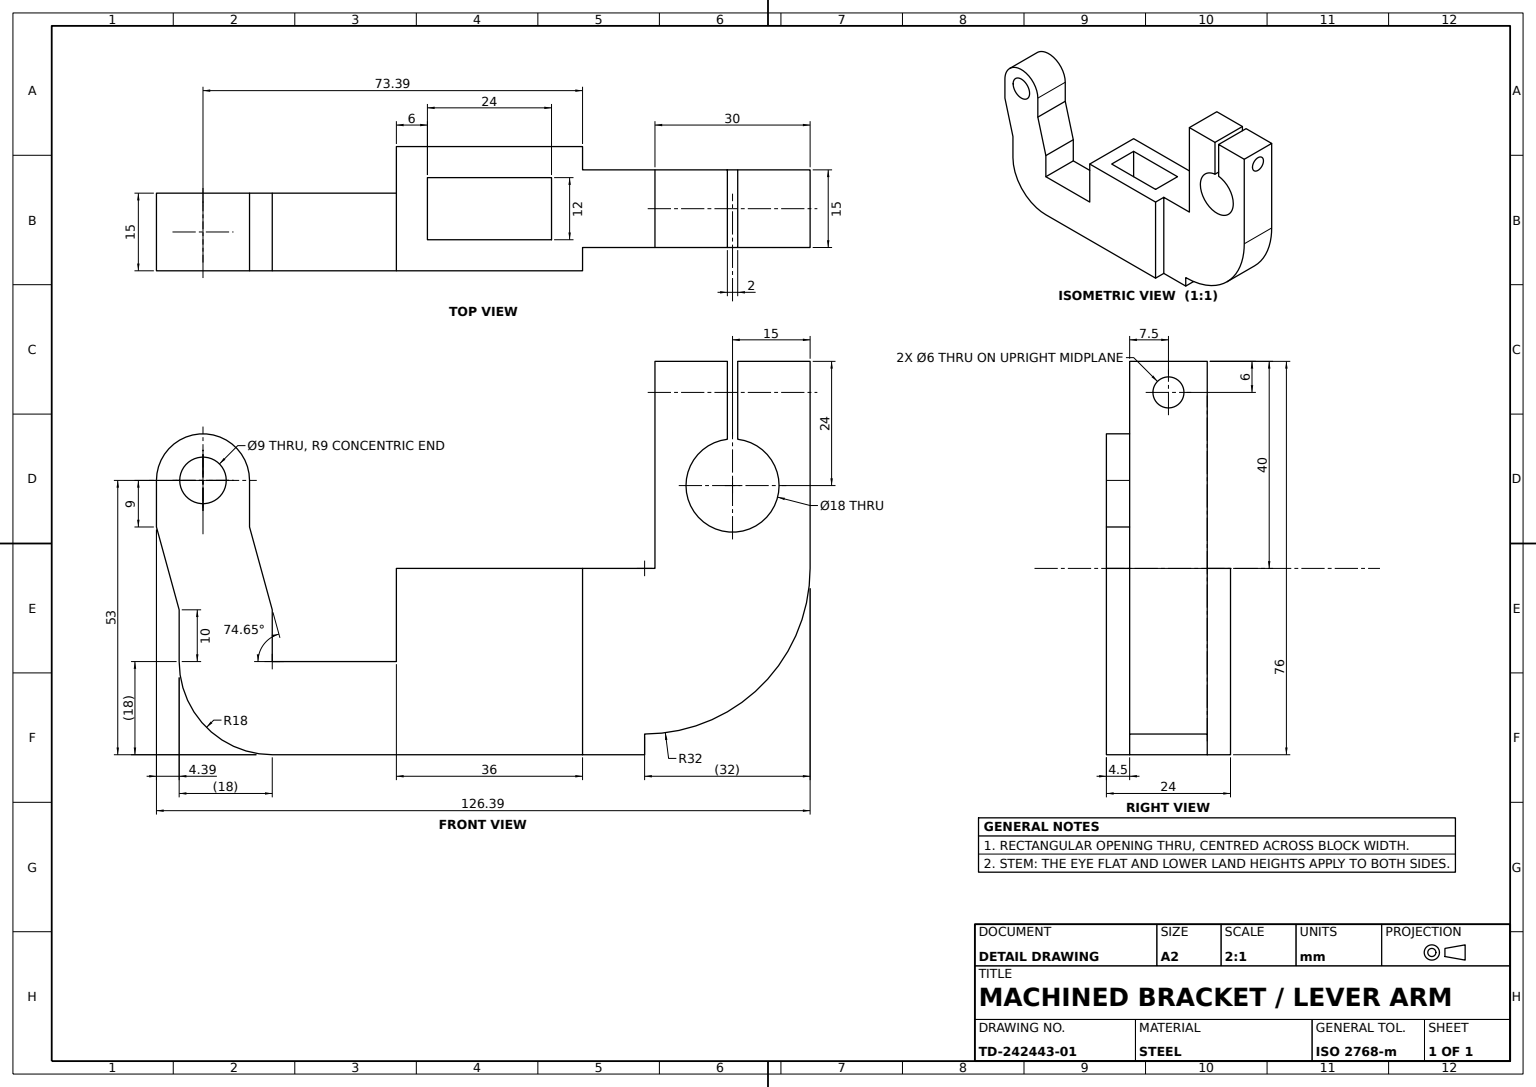
from build123d import *

# Parameters (mm, degrees)
BASE_BLOCK_SKETCH_W                = 36
BASE_BLOCK_SKETCH_H                = 24
BASE_BLOCK_DEPTH                   = 36
RECTANGULAR_POCKET_12X6_DEPTH      = 43
RECTANGULAR_POCKET_12X6_DEPTH_BACK = 43
RECTANGULAR_POCKET_SKETCH_W        = 24
RECTANGULAR_POCKET_SKETCH_H        = 12
CLAMP_UPRIGHT_SKETCH_W             = 12
CLAMP_UPRIGHT_SKETCH_H             = 15
CLAMP_UPRIGHT_DEPTH                = 36
CURVED_ARM_DEPTH                   = 15
CLAMP_BLOCK_SKETCH_W               = 30
CLAMP_BLOCK_SKETCH_H               = 15
CLAMP_BLOCK_DEPTH                  = 40
CLAMP_SPLIT_SLOT_1MM_DEPTH         = 101.001249992
CLAMP_SPLIT_SLOT_1MM_DEPTH_BACK    = 101.001249992
CLAMP_CROSS_HOLE_DEPTH             = 111.995495404
CLAMP_CROSS_HOLE_DEPTH_BACK        = 111.995495404
CROSS_HOLE_SKETCH_R                = 3
SIDE_START                         = -18
SIDE_LUG_SKETCH_W                  = 24
SIDE_LUG_SKETCH_H                  = 15
SIDE_LUG_DEPTH                     = 18
ARM_SEGMENT_DEPTH                  = 15
ARM_LINK_DEPTH                     = 15
PIVOT_EYE_SKETCH_R                 = 4.5
PIVOT_EYE_DEPTH                    = 15


with BuildPart() as part:
    # Base Block Sketch → Base Block (new body)
    with BuildSketch(Plane(origin=(0, 0, 0), x_dir=(1, 0, 0), z_dir=(0, 1, 0))):
        Rectangle(BASE_BLOCK_SKETCH_W, BASE_BLOCK_SKETCH_H)
    extrude(amount=BASE_BLOCK_DEPTH)

    # Rectangular Pocket Sketch → Rectangular Pocket 12x6 (cut, two sides: drawn at the far end of the back side and taken through both)
    with BuildSketch(Plane(origin=(0, 36, 0), x_dir=(1, 0, 0), z_dir=(0, 1, 0)).offset(-RECTANGULAR_POCKET_12X6_DEPTH_BACK)):
        Rectangle(RECTANGULAR_POCKET_SKETCH_W, RECTANGULAR_POCKET_SKETCH_H)
    extrude(amount=RECTANGULAR_POCKET_12X6_DEPTH + RECTANGULAR_POCKET_12X6_DEPTH_BACK, mode=Mode.SUBTRACT)

    # Clamp Upright Sketch → Clamp Upright (add)
    with BuildSketch(Plane(origin=(0, 36, 0), x_dir=(1, 0, 0), z_dir=(0, 1, 0))):
        with Locations((24, 0)):
            Rectangle(CLAMP_UPRIGHT_SKETCH_W, CLAMP_UPRIGHT_SKETCH_H)
    extrude(amount=-CLAMP_UPRIGHT_DEPTH)

    # Curved Arm Sketch → Curved Arm (add)
    with BuildSketch(Plane.XY.offset(7.5)):
        with BuildLine():
            Line((30, 36), (62, 36))
            ThreePointArc((62, 36), (52.627416998, 13.372583002), (30, 4))
            Line((30, 4), (30, 36))
        make_face()
    extrude(amount=-CURVED_ARM_DEPTH)

    # Clamp Block Sketch → Clamp Block (add)
    with BuildSketch(Plane(origin=(0, 36, 0), x_dir=(1, 0, 0), z_dir=(0, 1, 0))):
        with Locations((47, 0)):
            Rectangle(CLAMP_BLOCK_SKETCH_W, CLAMP_BLOCK_SKETCH_H)
    extrude(amount=CLAMP_BLOCK_DEPTH)

    # Clamp Split Slot Sketch → Clamp Split Slot 1mm (cut, two sides: drawn at the far end of the back side and taken through both)
    with BuildSketch(Plane.XY.offset(7.5).offset(-CLAMP_SPLIT_SLOT_1MM_DEPTH_BACK)):
        with BuildLine():
            Line((46, 76), (46, 60.94427191))
            ThreePointArc((46, 60.94427191), (47, 43), (48, 60.94427191))
            Line((48, 60.94427191), (48, 76))
            Line((48, 76), (46, 76))
        make_face()
    extrude(amount=CLAMP_SPLIT_SLOT_1MM_DEPTH + CLAMP_SPLIT_SLOT_1MM_DEPTH_BACK, mode=Mode.SUBTRACT)

    # Cross Hole Sketch → Clamp Cross Hole (cut, two sides: drawn at the far end of the back side and taken through both)
    with BuildSketch(Plane(origin=(62, 0, 0), x_dir=(0, 0, -1), z_dir=(1, 0, 0)).offset(-CLAMP_CROSS_HOLE_DEPTH_BACK)):
        with Locations((0, 70)):
            Circle(CROSS_HOLE_SKETCH_R)
    extrude(amount=CLAMP_CROSS_HOLE_DEPTH + CLAMP_CROSS_HOLE_DEPTH_BACK, mode=Mode.SUBTRACT)

    # Side Lug Sketch → Side Lug (add)
    with BuildSketch(Plane(origin=(0, 36, 0), x_dir=(1, 0, 0), z_dir=(0, 1, 0)).offset(SIDE_START)):
        with Locations((-30, -4.5)):
            Rectangle(SIDE_LUG_SKETCH_W, SIDE_LUG_SKETCH_H)
    extrude(amount=-SIDE_LUG_DEPTH)

    # Arm Segment Sketch → Arm Segment (add)
    with BuildSketch(Plane.XY.offset(12)):
        with BuildLine():
            Line((-42, 18), (-42, 28))
            Line((-42, 28), (-60, 28))
            Line((-60, 28), (-60, 18))
            ThreePointArc((-60, 18), (-54.727922061, 5.272077939), (-42, 0))
            Line((-42, 0), (-42, 18))
        make_face()
    extrude(amount=-ARM_SEGMENT_DEPTH)

    # Arm Link Sketch → Arm Link (add)
    with BuildSketch(Plane.XY.offset(12)):
        Polygon((-60, 28), (-42, 28), (-46.393085021, 44), (-64.393085021, 44), align=None)
    extrude(amount=-ARM_LINK_DEPTH)

    # Pivot Eye Sketch → Pivot Eye (add)
    with BuildSketch(Plane.XY.offset(12)):
        with BuildLine():
            Line((-64.393085021, 44), (-64.393085021, 53))
            ThreePointArc((-64.393085021, 53), (-55.393085021, 62), (-46.393085021, 53))
            Line((-46.393085021, 53), (-46.393085021, 44))
            Line((-46.393085021, 44), (-64.393085021, 44))
        make_face()
        with Locations((-55.393085021, 53)):
            Circle(PIVOT_EYE_SKETCH_R, mode=Mode.SUBTRACT)
    extrude(amount=-PIVOT_EYE_DEPTH)


solid = part.part
